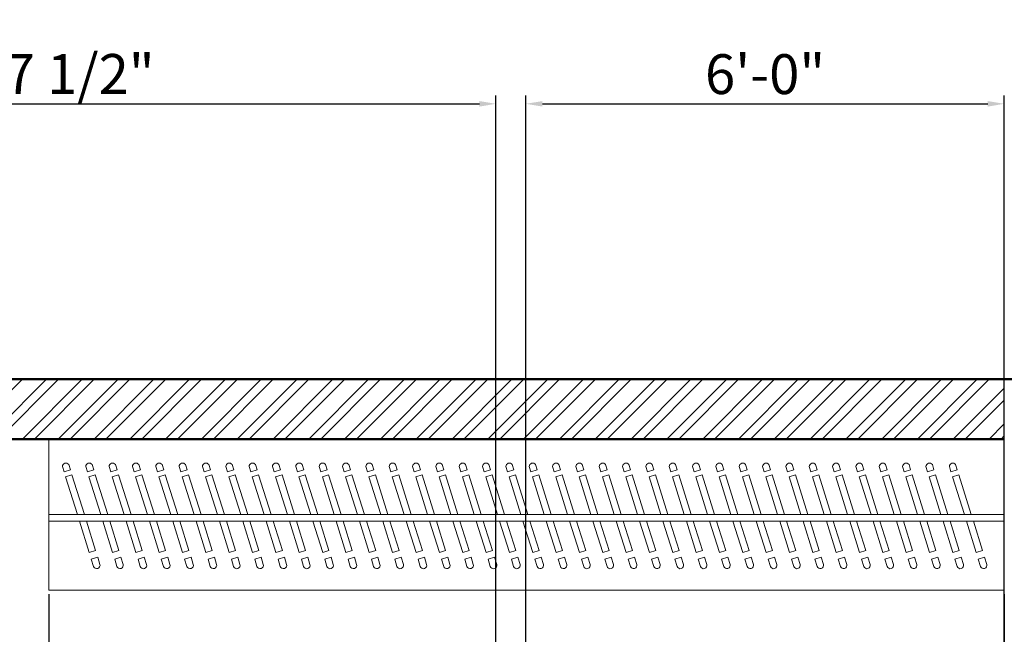
# Model space of a CAD drawing. Units: millimetres. Extents: x 20768 to 23556, y 50760 to 52704.
# Tile 28 of 36: x 21403 to 21551, y 52484 to 52577. Entities that reach past the tile are written whole.
import ezdxf

# ---------------------------------------------------------------- set-up
doc = ezdxf.new("R2010")
doc.units = ezdxf.units.MM
for name, color, linetype, lineweight in [('A-FURN', 8, 'Continuous', 18), ('A-WALL', 7, 'Continuous', 50), ('A-WALL-PATT', 8, 'Continuous', 13), ('S-ANNO-DIMS', 2, 'Continuous', 18)]:
    doc.layers.add(name, color=color, linetype=linetype, lineweight=lineweight)
doc.styles.get("Standard").update_dxf_attribs({"font": 'arial.ttf'})
doc.dimstyles.new('ISO-25', dxfattribs={"dimtxt": 6, "dimasz": 2.5, "dimexe": 1.25, "dimexo": 0.625, "dimtad": 1, "dimdec": 0, "dimlunit": 3, "dimtxsty": 'Standard', "dimcen": 2.5, "dimadec": 0, "dimazin": 0, "dimtfac": 1, "dimtdec": 0, "dimtmove": 0, "dimatfit": 3, "dimfxl": 1, "dimarcsym": 0})

# ---------------------------------------------------------------- blocks, each defined once
blk = doc.blocks.new('wb')
for p, q in [((21205.25, 52502.52), (21061.44, 52502.52)), ((21205.25, 52501.52), (21061.44, 52501.52))]:
    blk.add_line(p, q)
blk.add_lwpolyline([(21205.25, 52513.9), (21061.44, 52513.9), (21061.44, 52491.15), (21205.25, 52491.15)], close=True)
for points in [[(21064.45, 52510.07, 0.695903), (21063.5, 52509.77), (21063.75, 52508.98), (21064.7, 52509.27)], [(21067.97, 52510.07, 0.695903), (21067.01, 52509.77), (21067.26, 52508.98), (21068.21, 52509.27)], [(21071.48, 52510.07, 0.695903), (21070.52, 52509.77), (21070.77, 52508.98), (21071.73, 52509.27)], [(21074.99, 52510.07, 0.695903), (21074.04, 52509.77), (21074.28, 52508.98), (21075.24, 52509.27)], [(21078.5, 52510.07, 0.695903), (21077.55, 52509.77), (21077.8, 52508.98), (21078.75, 52509.27)], [(21082.02, 52510.07, 0.695903), (21081.06, 52509.77), (21081.31, 52508.98), (21082.26, 52509.27)], [(21085.53, 52510.07, 0.695903), (21084.57, 52509.77), (21084.82, 52508.98), (21085.78, 52509.27)], [(21089.04, 52510.07, 0.695903), (21088.09, 52509.77), (21088.33, 52508.98), (21089.29, 52509.27)], [(21092.55, 52510.07, 0.695903), (21091.6, 52509.77), (21091.85, 52508.98), (21092.8, 52509.27)], [(21096.07, 52510.07, 0.695903), (21095.11, 52509.77), (21095.36, 52508.98), (21096.31, 52509.27)], [(21099.58, 52510.07, 0.695903), (21098.62, 52509.77), (21098.87, 52508.98), (21099.83, 52509.27)], [(21103.09, 52510.07, 0.695903), (21102.14, 52509.77), (21102.38, 52508.98), (21103.34, 52509.27)], [(21106.6, 52510.07, 0.695903), (21105.65, 52509.77), (21105.9, 52508.98), (21106.85, 52509.27)], [(21110.12, 52510.07, 0.695903), (21109.16, 52509.77), (21109.41, 52508.98), (21110.36, 52509.27)], [(21113.63, 52510.07, 0.695903), (21112.67, 52509.77), (21112.92, 52508.98), (21113.88, 52509.27)], [(21117.14, 52510.07, 0.695903), (21116.19, 52509.77), (21116.43, 52508.98), (21117.39, 52509.27)], [(21120.65, 52510.07, 0.695903), (21119.7, 52509.77), (21119.95, 52508.98), (21120.9, 52509.27)], [(21124.17, 52510.07, 0.695903), (21123.21, 52509.77), (21123.46, 52508.98), (21124.41, 52509.27)], [(21127.68, 52510.07, 0.695903), (21126.72, 52509.77), (21126.97, 52508.98), (21127.93, 52509.27)], [(21131.19, 52510.07, 0.695903), (21130.24, 52509.77), (21130.48, 52508.98), (21131.44, 52509.27)], [(21134.7, 52510.07, 0.695903), (21133.75, 52509.77), (21134, 52508.98), (21134.95, 52509.27)], [(21138.22, 52510.07, 0.695903), (21137.26, 52509.77), (21137.51, 52508.98), (21138.46, 52509.27)], [(21141.73, 52510.07, 0.695903), (21140.77, 52509.77), (21141.02, 52508.98), (21141.98, 52509.27)], [(21145.24, 52510.07, 0.695903), (21144.29, 52509.77), (21144.54, 52508.98), (21145.49, 52509.27)], [(21148.75, 52510.07, 0.695903), (21147.8, 52509.77), (21148.05, 52508.98), (21149, 52509.27)], [(21152.27, 52510.07, 0.695903), (21151.31, 52509.77), (21151.56, 52508.98), (21152.52, 52509.27)], [(21155.78, 52510.07, 0.695903), (21154.83, 52509.77), (21155.07, 52508.98), (21156.03, 52509.27)], [(21159.29, 52510.07, 0.695903), (21158.34, 52509.77), (21158.59, 52508.98), (21159.54, 52509.27)], [(21162.8, 52510.07, 0.695903), (21161.85, 52509.77), (21162.1, 52508.98), (21163.05, 52509.27)], [(21166.32, 52510.07, 0.695903), (21165.36, 52509.77), (21165.61, 52508.98), (21166.57, 52509.27)], [(21169.83, 52510.07, 0.695903), (21168.88, 52509.77), (21169.12, 52508.98), (21170.08, 52509.27)], [(21173.34, 52510.07, 0.695903), (21172.39, 52509.77), (21172.64, 52508.98), (21173.59, 52509.27)], [(21176.86, 52510.07, 0.695903), (21175.9, 52509.77), (21176.15, 52508.98), (21177.1, 52509.27)], [(21180.37, 52510.07, 0.695903), (21179.41, 52509.77), (21179.66, 52508.98), (21180.62, 52509.27)], [(21183.88, 52510.07, 0.695903), (21182.93, 52509.77), (21183.17, 52508.98), (21184.13, 52509.27)], [(21187.39, 52510.07, 0.695903), (21186.44, 52509.77), (21186.69, 52508.98), (21187.64, 52509.27)], [(21190.91, 52510.07, 0.695903), (21189.95, 52509.77), (21190.2, 52508.98), (21191.15, 52509.27)], [(21194.42, 52510.07, 0.695903), (21193.46, 52509.77), (21193.71, 52508.98), (21194.67, 52509.27)], [(21197.93, 52510.07, 0.695903), (21196.98, 52509.77), (21197.22, 52508.98), (21198.18, 52509.27)], [(21068.81, 52496.1), (21067.85, 52495.8), (21068.19, 52494.73, 1), (21069.14, 52495.03)], [(21072.32, 52496.1), (21071.37, 52495.8), (21071.7, 52494.73, 1), (21072.65, 52495.03)], [(21075.83, 52496.1), (21074.88, 52495.8), (21075.21, 52494.73, 1), (21076.17, 52495.03)], [(21079.35, 52496.1), (21078.39, 52495.8), (21078.73, 52494.73, 1), (21079.68, 52495.03)], [(21082.86, 52496.1), (21081.9, 52495.8), (21082.24, 52494.73, 1), (21083.19, 52495.03)], [(21086.37, 52496.1), (21085.42, 52495.8), (21085.75, 52494.73, 1), (21086.7, 52495.03)], [(21089.88, 52496.1), (21088.93, 52495.8), (21089.26, 52494.73, 1), (21090.22, 52495.03)], [(21093.4, 52496.1), (21092.44, 52495.8), (21092.78, 52494.73, 1), (21093.73, 52495.03)], [(21096.91, 52496.1), (21095.95, 52495.8), (21096.29, 52494.73, 1), (21097.24, 52495.03)], [(21100.42, 52496.1), (21099.47, 52495.8), (21099.8, 52494.73, 1), (21100.76, 52495.03)], [(21103.93, 52496.1), (21102.98, 52495.8), (21103.31, 52494.73, 1), (21104.27, 52495.03)], [(21107.45, 52496.1), (21106.49, 52495.8), (21106.83, 52494.73, 1), (21107.78, 52495.03)], [(21110.96, 52496.1), (21110, 52495.8), (21110.34, 52494.73, 1), (21111.29, 52495.03)], [(21114.47, 52496.1), (21113.52, 52495.8), (21113.85, 52494.73, 1), (21114.81, 52495.03)], [(21117.98, 52496.1), (21117.03, 52495.8), (21117.36, 52494.73, 1), (21118.32, 52495.03)], [(21121.5, 52496.1), (21120.54, 52495.8), (21120.88, 52494.73, 1), (21121.83, 52495.03)], [(21125.01, 52496.1), (21124.05, 52495.8), (21124.39, 52494.73, 1), (21125.34, 52495.03)], [(21128.52, 52496.1), (21127.57, 52495.8), (21127.9, 52494.73, 1), (21128.86, 52495.03)], [(21132.03, 52496.1), (21131.08, 52495.8), (21131.41, 52494.73, 1), (21132.37, 52495.03)], [(21135.55, 52496.1), (21134.59, 52495.8), (21134.93, 52494.73, 1), (21135.88, 52495.03)], [(21139.06, 52496.1), (21138.1, 52495.8), (21138.44, 52494.73, 1), (21139.39, 52495.03)], [(21142.57, 52496.1), (21141.62, 52495.8), (21141.95, 52494.73, 1), (21142.91, 52495.03)], [(21146.08, 52496.1), (21145.13, 52495.8), (21145.46, 52494.73, 1), (21146.42, 52495.03)], [(21149.6, 52496.1), (21148.64, 52495.8), (21148.98, 52494.73, 1), (21149.93, 52495.03)], [(21153.11, 52496.1), (21152.15, 52495.8), (21152.49, 52494.73, 1), (21153.44, 52495.03)], [(21156.62, 52496.1), (21155.67, 52495.8), (21156, 52494.73, 1), (21156.96, 52495.03)], [(21160.13, 52496.1), (21159.18, 52495.8), (21159.51, 52494.73, 1), (21160.47, 52495.03)], [(21163.65, 52496.1), (21162.69, 52495.8), (21163.03, 52494.73, 1), (21163.98, 52495.03)], [(21167.16, 52496.1), (21166.2, 52495.8), (21166.54, 52494.73, 1), (21167.49, 52495.03)], [(21170.67, 52496.1), (21169.72, 52495.8), (21170.05, 52494.73, 1), (21171.01, 52495.03)], [(21174.18, 52496.1), (21173.23, 52495.8), (21173.56, 52494.73, 1), (21174.52, 52495.03)], [(21177.7, 52496.1), (21176.74, 52495.8), (21177.08, 52494.73, 1), (21178.03, 52495.03)], [(21181.21, 52496.1), (21180.25, 52495.8), (21180.59, 52494.73, 1), (21181.54, 52495.03)], [(21184.72, 52496.1), (21183.77, 52495.8), (21184.1, 52494.73, 1), (21185.06, 52495.03)], [(21188.23, 52496.1), (21187.28, 52495.8), (21187.61, 52494.73, 1), (21188.57, 52495.03)], [(21191.75, 52496.1), (21190.79, 52495.8), (21191.13, 52494.73, 1), (21192.08, 52495.03)], [(21195.26, 52496.1), (21194.31, 52495.8), (21194.64, 52494.73, 1), (21195.59, 52495.03)], [(21198.77, 52496.1), (21197.82, 52495.8), (21198.15, 52494.73, 1), (21199.11, 52495.03)], [(21202.29, 52496.1), (21201.33, 52495.8), (21201.67, 52494.73, 1), (21202.62, 52495.03)]]:
    blk.add_lwpolyline(points, format="xyb", close=True)
for points in [[(21065.76, 52502.52), (21063.98, 52508.23), (21064.93, 52508.53), (21066.81, 52502.52)], [(21069.27, 52502.52), (21067.49, 52508.23), (21068.44, 52508.53), (21070.32, 52502.52)], [(21072.78, 52502.52), (21071, 52508.23), (21071.96, 52508.53), (21073.83, 52502.52)], [(21076.3, 52502.52), (21074.51, 52508.23), (21075.47, 52508.53), (21077.34, 52502.52)], [(21079.81, 52502.52), (21078.03, 52508.23), (21078.98, 52508.53), (21080.86, 52502.52)], [(21083.32, 52502.52), (21081.54, 52508.23), (21082.49, 52508.53), (21084.37, 52502.52)], [(21086.83, 52502.52), (21085.05, 52508.23), (21086.01, 52508.53), (21087.88, 52502.52)], [(21090.35, 52502.52), (21088.57, 52508.23), (21089.52, 52508.53), (21091.39, 52502.52)], [(21093.86, 52502.52), (21092.08, 52508.23), (21093.03, 52508.53), (21094.91, 52502.52)], [(21097.37, 52502.52), (21095.59, 52508.23), (21096.55, 52508.53), (21098.42, 52502.52)], [(21100.88, 52502.52), (21099.1, 52508.23), (21100.06, 52508.53), (21101.93, 52502.52)], [(21104.4, 52502.52), (21102.62, 52508.23), (21103.57, 52508.53), (21105.44, 52502.52)], [(21107.91, 52502.52), (21106.13, 52508.23), (21107.08, 52508.53), (21108.96, 52502.52)], [(21111.42, 52502.52), (21109.64, 52508.23), (21110.6, 52508.53), (21112.47, 52502.52)], [(21114.93, 52502.52), (21113.15, 52508.23), (21114.11, 52508.53), (21115.98, 52502.52)], [(21118.45, 52502.52), (21116.67, 52508.23), (21117.62, 52508.53), (21119.49, 52502.52)], [(21121.96, 52502.52), (21120.18, 52508.23), (21121.13, 52508.53), (21123.01, 52502.52)], [(21125.47, 52502.52), (21123.69, 52508.23), (21124.65, 52508.53), (21126.52, 52502.52)], [(21128.98, 52502.52), (21127.2, 52508.23), (21128.16, 52508.53), (21130.03, 52502.52)], [(21132.5, 52502.52), (21130.72, 52508.23), (21131.67, 52508.53), (21133.54, 52502.52)], [(21136.01, 52502.52), (21134.23, 52508.23), (21135.18, 52508.53), (21137.06, 52502.52)], [(21139.52, 52502.52), (21137.74, 52508.23), (21138.7, 52508.53), (21140.57, 52502.52)], [(21143.03, 52502.52), (21141.25, 52508.23), (21142.21, 52508.53), (21144.08, 52502.52)], [(21146.55, 52502.52), (21144.77, 52508.23), (21145.72, 52508.53), (21147.59, 52502.52)], [(21150.06, 52502.52), (21148.28, 52508.23), (21149.23, 52508.53), (21151.11, 52502.52)], [(21153.57, 52502.52), (21151.79, 52508.23), (21152.75, 52508.53), (21154.62, 52502.52)], [(21157.08, 52502.52), (21155.3, 52508.23), (21156.26, 52508.53), (21158.13, 52502.52)], [(21160.6, 52502.52), (21158.82, 52508.23), (21159.77, 52508.53), (21161.64, 52502.52)], [(21164.11, 52502.52), (21162.33, 52508.23), (21163.28, 52508.53), (21165.16, 52502.52)], [(21167.62, 52502.52), (21165.84, 52508.23), (21166.8, 52508.53), (21168.67, 52502.52)], [(21171.13, 52502.52), (21169.35, 52508.23), (21170.31, 52508.53), (21172.18, 52502.52)], [(21174.65, 52502.52), (21172.87, 52508.23), (21173.82, 52508.53), (21175.69, 52502.52)], [(21178.16, 52502.52), (21176.38, 52508.23), (21177.33, 52508.53), (21179.21, 52502.52)], [(21181.67, 52502.52), (21179.89, 52508.23), (21180.85, 52508.53), (21182.72, 52502.52)], [(21185.19, 52502.52), (21183.4, 52508.23), (21184.36, 52508.53), (21186.23, 52502.52)], [(21188.7, 52502.52), (21186.92, 52508.23), (21187.87, 52508.53), (21189.75, 52502.52)], [(21192.21, 52502.52), (21190.43, 52508.23), (21191.38, 52508.53), (21193.26, 52502.52)], [(21195.72, 52502.52), (21193.94, 52508.23), (21194.9, 52508.53), (21196.77, 52502.52)], [(21199.24, 52502.52), (21197.46, 52508.23), (21198.41, 52508.53), (21200.28, 52502.52)], [(21066.07, 52501.52), (21067.54, 52496.81), (21068.49, 52497.1), (21067.12, 52501.52)], [(21069.58, 52501.52), (21071.05, 52496.81), (21072.01, 52497.1), (21070.63, 52501.52)], [(21073.09, 52501.52), (21074.57, 52496.81), (21075.52, 52497.1), (21074.14, 52501.52)], [(21076.61, 52501.52), (21078.08, 52496.81), (21079.03, 52497.1), (21077.65, 52501.52)], [(21080.12, 52501.52), (21081.59, 52496.81), (21082.55, 52497.1), (21081.17, 52501.52)], [(21083.63, 52501.52), (21085.1, 52496.81), (21086.06, 52497.1), (21084.68, 52501.52)], [(21087.14, 52501.52), (21088.62, 52496.81), (21089.57, 52497.1), (21088.19, 52501.52)], [(21090.66, 52501.52), (21092.13, 52496.81), (21093.08, 52497.1), (21091.7, 52501.52)], [(21094.17, 52501.52), (21095.64, 52496.81), (21096.6, 52497.1), (21095.22, 52501.52)], [(21097.68, 52501.52), (21099.15, 52496.81), (21100.11, 52497.1), (21098.73, 52501.52)], [(21101.2, 52501.52), (21102.67, 52496.81), (21103.62, 52497.1), (21102.24, 52501.52)], [(21104.71, 52501.52), (21106.18, 52496.81), (21107.13, 52497.1), (21105.76, 52501.52)], [(21108.22, 52501.52), (21109.69, 52496.81), (21110.65, 52497.1), (21109.27, 52501.52)], [(21111.73, 52501.52), (21113.2, 52496.81), (21114.16, 52497.1), (21112.78, 52501.52)], [(21115.25, 52501.52), (21116.72, 52496.81), (21117.67, 52497.1), (21116.29, 52501.52)], [(21118.76, 52501.52), (21120.23, 52496.81), (21121.18, 52497.1), (21119.81, 52501.52)], [(21122.27, 52501.52), (21123.74, 52496.81), (21124.7, 52497.1), (21123.32, 52501.52)], [(21125.78, 52501.52), (21127.25, 52496.81), (21128.21, 52497.1), (21126.83, 52501.52)], [(21129.3, 52501.52), (21130.77, 52496.81), (21131.72, 52497.1), (21130.34, 52501.52)], [(21132.81, 52501.52), (21134.28, 52496.81), (21135.23, 52497.1), (21133.86, 52501.52)], [(21136.32, 52501.52), (21137.79, 52496.81), (21138.75, 52497.1), (21137.37, 52501.52)], [(21139.83, 52501.52), (21141.3, 52496.81), (21142.26, 52497.1), (21140.88, 52501.52)], [(21143.35, 52501.52), (21144.82, 52496.81), (21145.77, 52497.1), (21144.39, 52501.52)], [(21146.86, 52501.52), (21148.33, 52496.81), (21149.28, 52497.1), (21147.91, 52501.52)], [(21150.37, 52501.52), (21151.84, 52496.81), (21152.8, 52497.1), (21151.42, 52501.52)], [(21153.88, 52501.52), (21155.35, 52496.81), (21156.31, 52497.1), (21154.93, 52501.52)], [(21157.4, 52501.52), (21158.87, 52496.81), (21159.82, 52497.1), (21158.44, 52501.52)], [(21160.91, 52501.52), (21162.38, 52496.81), (21163.33, 52497.1), (21161.96, 52501.52)], [(21164.42, 52501.52), (21165.89, 52496.81), (21166.85, 52497.1), (21165.47, 52501.52)], [(21167.93, 52501.52), (21169.4, 52496.81), (21170.36, 52497.1), (21168.98, 52501.52)], [(21171.45, 52501.52), (21172.92, 52496.81), (21173.87, 52497.1), (21172.49, 52501.52)], [(21174.96, 52501.52), (21176.43, 52496.81), (21177.38, 52497.1), (21176.01, 52501.52)], [(21178.47, 52501.52), (21179.94, 52496.81), (21180.9, 52497.1), (21179.52, 52501.52)], [(21181.98, 52501.52), (21183.46, 52496.81), (21184.41, 52497.1), (21183.03, 52501.52)], [(21185.5, 52501.52), (21186.97, 52496.81), (21187.92, 52497.1), (21186.54, 52501.52)], [(21189.01, 52501.52), (21190.48, 52496.81), (21191.43, 52497.1), (21190.06, 52501.52)], [(21192.52, 52501.52), (21193.99, 52496.81), (21194.95, 52497.1), (21193.57, 52501.52)], [(21196.03, 52501.52), (21197.51, 52496.81), (21198.46, 52497.1), (21197.08, 52501.52)], [(21199.55, 52501.52), (21201.02, 52496.81), (21201.97, 52497.1), (21200.59, 52501.52)]]:
    blk.add_lwpolyline(points)
blk = doc.blocks.new('*D187')
at = {"layer": 'Defpoints', "color": 0, "transparency": 16777216}
for p in [(21406.93, 52491.15), (21550.74, 52491.15), (21550.74, 52469.58)]:
    blk.add_point(p, dxfattribs=at)
at = {"layer": 'S-ANNO-DIMS', "color": 0, "lineweight": -2, "transparency": 16777216}
for p, q in [((21406.93, 52490.53), (21406.93, 52468.33)), ((21550.74, 52490.53), (21550.74, 52468.33)), ((21409.43, 52469.58), (21548.24, 52469.58))]:
    blk.add_line(p, q, dxfattribs=at)
at = {"layer": 'S-ANNO-DIMS', "color": 0, "transparency": 16777216}
for points in [[(21409.43, 52470), (21409.43, 52469.16), (21406.93, 52469.58)], [(21548.24, 52470), (21548.24, 52469.16), (21550.74, 52469.58)]]:
    blk.add_solid(points, dxfattribs=at)
at = {"layer": 'S-ANNO-DIMS', "color": 0, "transparency": 16777216, "insert": (21478.84, 52473.31), "char_height": 6, "attachment_point": 5}
blk.add_mtext('WARDROBE 12\'-0" TYP.', dxfattribs=at)
blk = doc.blocks.new('*D215')
at = {"layer": 'Defpoints', "color": 0, "transparency": 16777216}
for p in [(21474.24, 52564.4), (21334.74, 52329.4), (21474.24, 52329.4)]:
    blk.add_point(p, dxfattribs=at)
at = {"layer": 'S-ANNO-DIMS', "color": 0, "lineweight": -2, "transparency": 16777216}
for p, q in [((21334.74, 52330.02), (21334.74, 52565.65)), ((21337.24, 52564.4), (21471.74, 52564.4)), ((21474.24, 52330.02), (21474.24, 52565.65))]:
    blk.add_line(p, q, dxfattribs=at)
at = {"layer": 'S-ANNO-DIMS', "color": 0, "transparency": 16777216}
for points in [[(21337.24, 52564.81), (21337.24, 52563.98), (21334.74, 52564.4)], [(21471.74, 52564.81), (21471.74, 52563.98), (21474.24, 52564.4)]]:
    blk.add_solid(points, dxfattribs=at)
at = {"layer": 'S-ANNO-DIMS', "color": 0, "transparency": 16777216, "insert": (21404.49, 52568.12), "char_height": 6, "attachment_point": 5}
blk.add_mtext('11\'-7 1/2"', dxfattribs=at)
blk = doc.blocks.new('*D216')
at = {"layer": 'Defpoints', "color": 0, "transparency": 16777216}
for p in [(21550.74, 52564.4), (21478.74, 52209.4), (21550.74, 52209.4)]:
    blk.add_point(p, dxfattribs=at)
at = {"layer": 'S-ANNO-DIMS', "color": 0, "lineweight": -2, "transparency": 16777216}
for p, q in [((21478.74, 52210.02), (21478.74, 52565.65)), ((21481.24, 52564.4), (21548.24, 52564.4)), ((21550.74, 52210.02), (21550.74, 52565.65))]:
    blk.add_line(p, q, dxfattribs=at)
at = {"layer": 'S-ANNO-DIMS', "color": 0, "transparency": 16777216}
for points in [[(21481.24, 52564.81), (21481.24, 52563.98), (21478.74, 52564.4)], [(21548.24, 52564.81), (21548.24, 52563.98), (21550.74, 52564.4)]]:
    blk.add_solid(points, dxfattribs=at)
at = {"layer": 'S-ANNO-DIMS', "color": 0, "transparency": 16777216, "insert": (21514.74, 52568.09), "char_height": 6, "attachment_point": 5}
blk.add_mtext('6\'-0"', dxfattribs=at)

msp = doc.modelspace()

# ---------------------------------------------------------------- hatches: boundary and pattern name
at = {"layer": 'A-WALL-PATT'}
h = msp.add_hatch(dxfattribs=at)
h.set_pattern_fill('ANSI32', color=256, scale=0.4)
h.set_pattern_definition([(45, (-37.4434, 0), (-2.69407684, 2.69407684), []), (45, (-35.6473, 0), (-2.69407684, 2.69407684), [])])
h.paths.add_polyline_path([(21550.74, 52522.9), (21334.74, 52522.9), (21334.74, 52513.9), (21550.74, 52513.9)])

# ---------------------------------------------------------------- linework, layer by layer
at = {"layer": 'A-WALL'}
for p, q in [((21325.74, 52522.9), (21559.74, 52522.9)), ((21334.74, 52513.9), (21550.74, 52513.9))]:
    msp.add_line(p, q, dxfattribs=at)

# ---------------------------------------------------------------- block references
at = {"layer": 'A-FURN'}
msp.add_blockref('wb', (345.49, 0), dxfattribs=at)

# ---------------------------------------------------------------- dimensions: what is measured, and where the dimension line sits
at = {"layer": 'S-ANNO-DIMS'}
for base, p1, p2, picture, middle in [((21474.24, 52564.4), (21334.74, 52329.4), (21474.24, 52329.4), '*D215', (21404.49, 52568.12)), ((21550.74, 52564.4), (21478.74, 52209.4), (21550.74, 52209.4), '*D216', (21514.74, 52568.09))]:
    dim = msp.add_linear_dim(base=base, p1=p1, p2=p2, dimstyle='ISO-25', override={"dimdec": 1, "dimlfac": 1, "dimrnd": 0, "dimzin": 1, "dimdsep": 46, "dimlunit": 4, "dimfrac": 2}, dxfattribs=at)
    dim.commit()
    dim.dimension.update_dxf_attribs({"geometry": picture, "text_midpoint": middle})
dim = msp.add_linear_dim(base=(21550.74, 52469.58), p1=(21406.93, 52491.15), p2=(21550.74, 52491.15), text='WARDROBE <> TYP.', dimstyle='ISO-25', override={"dimdec": 1, "dimrnd": 0, "dimzin": 1, "dimlunit": 4, "dimfrac": 2}, dxfattribs=at)
dim.commit()
dim.dimension.update_dxf_attribs({"geometry": '*D187', "text_midpoint": (21478.84, 52473.31)})

doc.saveas('drawing.dxf')
